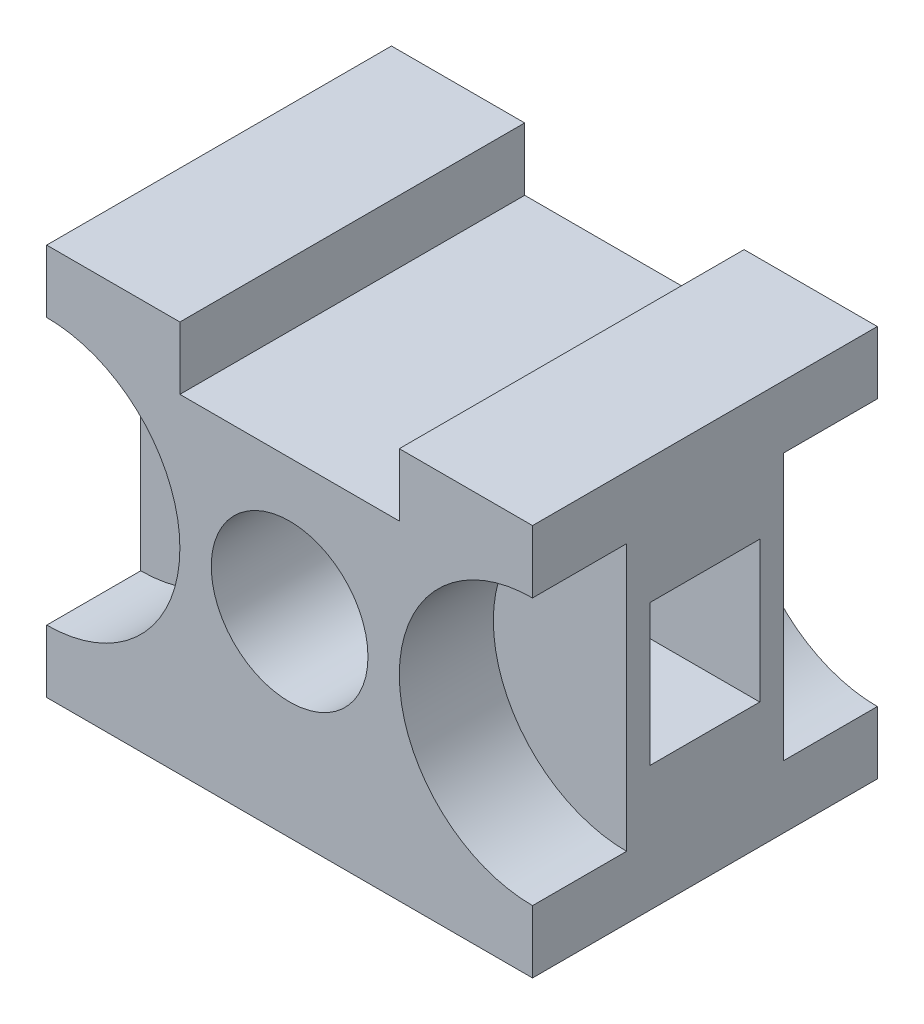
ISO-10303-21;
HEADER;
FILE_DESCRIPTION(('STEP AP214'),'2;1');
FILE_NAME('part.step','',(''),(''),'','','');
FILE_SCHEMA(('AUTOMOTIVE_DESIGN { 1 0 10303 214 1 1 1 1 }'));
ENDSEC;
DATA;
#1=APPLICATION_CONTEXT('core data for automotive mechanical design processes');
#2=APPLICATION_PROTOCOL_DEFINITION('international standard','automotive_design',2000,#1);
#3=PRODUCT_CONTEXT('',#1,'mechanical');
#4=PRODUCT('Part','Part','',(#3));
#5=PRODUCT_RELATED_PRODUCT_CATEGORY('part','',(#4));
#6=PRODUCT_DEFINITION_FORMATION('','',#4);
#7=PRODUCT_DEFINITION_CONTEXT('part definition',#1,'design');
#8=PRODUCT_DEFINITION('design','',#6,#7);
#9=PRODUCT_DEFINITION_SHAPE('','',#8);
#10=(LENGTH_UNIT() NAMED_UNIT(*) SI_UNIT(.MILLI.,.METRE.));
#11=(NAMED_UNIT(*) PLANE_ANGLE_UNIT() SI_UNIT($,.RADIAN.));
#12=(NAMED_UNIT(*) SI_UNIT($,.STERADIAN.) SOLID_ANGLE_UNIT());
#13=UNCERTAINTY_MEASURE_WITH_UNIT(LENGTH_MEASURE(1.E-05),#10,'distance_accuracy_value','');
#14=(GEOMETRIC_REPRESENTATION_CONTEXT(3) GLOBAL_UNCERTAINTY_ASSIGNED_CONTEXT((#13)) GLOBAL_UNIT_ASSIGNED_CONTEXT((#10,
#11,#12)) REPRESENTATION_CONTEXT('',''));
#15=CARTESIAN_POINT('',(0.,0.,0.));
#16=DIRECTION('',(0.,0.,1.));
#17=DIRECTION('',(1.,0.,0.));
#18=AXIS2_PLACEMENT_3D('',#15,#16,#17);
#19=CARTESIAN_POINT('',(-31.,25.,44.));
#20=DIRECTION('',(0.,-1.,0.));
#21=DIRECTION('',(0.,0.,-1.));
#22=AXIS2_PLACEMENT_3D('',#19,#20,#21);
#23=PLANE('',#22);
#24=DIRECTION('',(0.,0.,-1.));
#25=VECTOR('',#24,1.);
#26=CARTESIAN_POINT('',(14.,25.,172.743131660773));
#27=LINE('',#26,#25);
#28=CARTESIAN_POINT('',(14.,25.,44.));
#29=VERTEX_POINT('',#28);
#30=CARTESIAN_POINT('',(14.,25.,0.));
#31=VERTEX_POINT('',#30);
#32=EDGE_CURVE('E272',#29,#31,#27,.T.);
#33=ORIENTED_EDGE('',*,*,#32,.F.);
#34=DIRECTION('',(-1.,0.,0.));
#35=VECTOR('',#34,1.);
#36=CARTESIAN_POINT('',(-31.,25.,44.));
#37=LINE('',#36,#35);
#38=CARTESIAN_POINT('',(31.,25.,44.));
#39=VERTEX_POINT('',#38);
#40=EDGE_CURVE('E323',#39,#29,#37,.T.);
#41=ORIENTED_EDGE('',*,*,#40,.F.);
#42=DIRECTION('',(0.,0.,-1.));
#43=VECTOR('',#42,1.);
#44=CARTESIAN_POINT('',(31.,25.,44.));
#45=LINE('',#44,#43);
#46=CARTESIAN_POINT('',(31.,25.,0.));
#47=VERTEX_POINT('',#46);
#48=EDGE_CURVE('E358',#39,#47,#45,.T.);
#49=ORIENTED_EDGE('',*,*,#48,.T.);
#50=DIRECTION('',(-1.,0.,0.));
#51=VECTOR('',#50,1.);
#52=CARTESIAN_POINT('',(-31.,25.,0.));
#53=LINE('',#52,#51);
#54=EDGE_CURVE('E339',#47,#31,#53,.T.);
#55=ORIENTED_EDGE('',*,*,#54,.T.);
#56=EDGE_LOOP('',(#33,#41,#49,#55));
#57=FACE_BOUND('',#56,.T.);
#58=ADVANCED_FACE('F39',(#57),#23,.F.);
#59=CARTESIAN_POINT('',(0.,0.,44.));
#60=DIRECTION('',(0.,0.,-1.));
#61=DIRECTION('',(-1.,0.,0.));
#62=AXIS2_PLACEMENT_3D('',#59,#60,#61);
#63=PLANE('',#62);
#64=CARTESIAN_POINT('',(0.,0.,44.));
#65=DIRECTION('',(0.,0.,1.));
#66=DIRECTION('',(1.,0.,0.));
#67=AXIS2_PLACEMENT_3D('',#64,#65,#66);
#68=CIRCLE('',#67,10.);
#69=CARTESIAN_POINT('',(10.,0.,44.));
#70=VERTEX_POINT('',#69);
#71=EDGE_CURVE('E311',#70,#70,#68,.T.);
#72=ORIENTED_EDGE('',*,*,#71,.F.);
#73=EDGE_LOOP('',(#72));
#74=FACE_BOUND('',#73,.T.);
#75=DIRECTION('',(0.,-1.,0.));
#76=VECTOR('',#75,1.);
#77=CARTESIAN_POINT('',(-14.,0.,44.));
#78=LINE('',#77,#76);
#79=CARTESIAN_POINT('',(-14.,25.,44.));
#80=VERTEX_POINT('',#79);
#81=CARTESIAN_POINT('',(-14.,17.,44.));
#82=VERTEX_POINT('',#81);
#83=EDGE_CURVE('E281',#80,#82,#78,.T.);
#84=ORIENTED_EDGE('',*,*,#83,.F.);
#85=CARTESIAN_POINT('',(-31.,25.,44.));
#86=VERTEX_POINT('',#85);
#87=EDGE_CURVE('E324',#80,#86,#37,.T.);
#88=ORIENTED_EDGE('',*,*,#87,.T.);
#89=DIRECTION('',(0.,-1.,0.));
#90=VECTOR('',#89,1.);
#91=CARTESIAN_POINT('',(-31.,-25.,44.));
#92=LINE('',#91,#90);
#93=CARTESIAN_POINT('',(-31.,17.,44.));
#94=VERTEX_POINT('',#93);
#95=EDGE_CURVE('E330',#86,#94,#92,.T.);
#96=ORIENTED_EDGE('',*,*,#95,.T.);
#97=CARTESIAN_POINT('',(-31.,0.,44.));
#98=DIRECTION('',(0.,0.,1.));
#99=DIRECTION('',(-1.,0.,0.));
#100=AXIS2_PLACEMENT_3D('',#97,#98,#99);
#101=CIRCLE('',#100,17.);
#102=CARTESIAN_POINT('',(-31.,-17.,44.));
#103=VERTEX_POINT('',#102);
#104=EDGE_CURVE('E286',#103,#94,#101,.T.);
#105=ORIENTED_EDGE('',*,*,#104,.F.);
#106=CARTESIAN_POINT('',(-31.,-25.,44.));
#107=VERTEX_POINT('',#106);
#108=EDGE_CURVE('E327',#103,#107,#92,.T.);
#109=ORIENTED_EDGE('',*,*,#108,.T.);
#110=DIRECTION('',(1.,0.,0.));
#111=VECTOR('',#110,1.);
#112=CARTESIAN_POINT('',(-31.,-25.,44.));
#113=LINE('',#112,#111);
#114=CARTESIAN_POINT('',(31.,-25.,44.));
#115=VERTEX_POINT('',#114);
#116=EDGE_CURVE('E331',#107,#115,#113,.T.);
#117=ORIENTED_EDGE('',*,*,#116,.T.);
#118=DIRECTION('',(0.,1.,0.));
#119=VECTOR('',#118,1.);
#120=CARTESIAN_POINT('',(31.,-25.,44.));
#121=LINE('',#120,#119);
#122=CARTESIAN_POINT('',(31.,-17.,44.));
#123=VERTEX_POINT('',#122);
#124=EDGE_CURVE('E318',#115,#123,#121,.T.);
#125=ORIENTED_EDGE('',*,*,#124,.T.);
#126=CARTESIAN_POINT('',(31.,0.,44.));
#127=DIRECTION('',(0.,0.,1.));
#128=DIRECTION('',(1.,0.,0.));
#129=AXIS2_PLACEMENT_3D('',#126,#127,#128);
#130=CIRCLE('',#129,17.);
#131=CARTESIAN_POINT('',(31.,17.,44.));
#132=VERTEX_POINT('',#131);
#133=EDGE_CURVE('E296',#132,#123,#130,.T.);
#134=ORIENTED_EDGE('',*,*,#133,.F.);
#135=EDGE_CURVE('E321',#132,#39,#121,.T.);
#136=ORIENTED_EDGE('',*,*,#135,.T.);
#137=ORIENTED_EDGE('',*,*,#40,.T.);
#138=DIRECTION('',(0.,1.,0.));
#139=VECTOR('',#138,1.);
#140=CARTESIAN_POINT('',(14.,0.,44.));
#141=LINE('',#140,#139);
#142=CARTESIAN_POINT('',(14.,17.,44.));
#143=VERTEX_POINT('',#142);
#144=EDGE_CURVE('E283',#143,#29,#141,.T.);
#145=ORIENTED_EDGE('',*,*,#144,.F.);
#146=DIRECTION('',(1.,0.,0.));
#147=VECTOR('',#146,1.);
#148=CARTESIAN_POINT('',(0.,17.,44.));
#149=LINE('',#148,#147);
#150=EDGE_CURVE('E282',#82,#143,#149,.T.);
#151=ORIENTED_EDGE('',*,*,#150,.F.);
#152=EDGE_LOOP('',(#84,#88,#96,#105,#109,#117,#125,#134,#136,#137,#145,#151));
#153=FACE_BOUND('',#152,.T.);
#154=ADVANCED_FACE('F408',(#74,#153),#63,.F.);
#155=CARTESIAN_POINT('',(0.,0.,0.));
#156=DIRECTION('',(0.,0.,-1.));
#157=DIRECTION('',(-1.,0.,0.));
#158=AXIS2_PLACEMENT_3D('',#155,#156,#157);
#159=PLANE('',#158);
#160=CARTESIAN_POINT('',(31.,0.,0.));
#161=DIRECTION('',(0.,0.,-1.));
#162=DIRECTION('',(-1.,0.,0.));
#163=AXIS2_PLACEMENT_3D('',#160,#161,#162);
#164=CIRCLE('',#163,17.);
#165=CARTESIAN_POINT('',(31.,-17.,0.));
#166=VERTEX_POINT('',#165);
#167=CARTESIAN_POINT('',(31.,17.,0.));
#168=VERTEX_POINT('',#167);
#169=EDGE_CURVE('E245',#166,#168,#164,.T.);
#170=ORIENTED_EDGE('',*,*,#169,.F.);
#171=DIRECTION('',(0.,1.,0.));
#172=VECTOR('',#171,1.);
#173=CARTESIAN_POINT('',(31.,-25.,0.));
#174=LINE('',#173,#172);
#175=CARTESIAN_POINT('',(31.,-25.,0.));
#176=VERTEX_POINT('',#175);
#177=EDGE_CURVE('E332',#176,#166,#174,.T.);
#178=ORIENTED_EDGE('',*,*,#177,.F.);
#179=DIRECTION('',(1.,0.,0.));
#180=VECTOR('',#179,1.);
#181=CARTESIAN_POINT('',(-31.,-25.,0.));
#182=LINE('',#181,#180);
#183=CARTESIAN_POINT('',(-31.,-25.,0.));
#184=VERTEX_POINT('',#183);
#185=EDGE_CURVE('E348',#184,#176,#182,.T.);
#186=ORIENTED_EDGE('',*,*,#185,.F.);
#187=DIRECTION('',(0.,-1.,0.));
#188=VECTOR('',#187,1.);
#189=CARTESIAN_POINT('',(-31.,-25.,0.));
#190=LINE('',#189,#188);
#191=CARTESIAN_POINT('',(-31.,-17.,0.));
#192=VERTEX_POINT('',#191);
#193=EDGE_CURVE('E345',#192,#184,#190,.T.);
#194=ORIENTED_EDGE('',*,*,#193,.F.);
#195=CARTESIAN_POINT('',(-31.,0.,0.));
#196=DIRECTION('',(0.,0.,-1.));
#197=DIRECTION('',(-1.,0.,0.));
#198=AXIS2_PLACEMENT_3D('',#195,#196,#197);
#199=CIRCLE('',#198,17.);
#200=CARTESIAN_POINT('',(-31.,17.,0.));
#201=VERTEX_POINT('',#200);
#202=EDGE_CURVE('E259',#201,#192,#199,.T.);
#203=ORIENTED_EDGE('',*,*,#202,.F.);
#204=CARTESIAN_POINT('',(-31.,25.,0.));
#205=VERTEX_POINT('',#204);
#206=EDGE_CURVE('E344',#205,#201,#190,.T.);
#207=ORIENTED_EDGE('',*,*,#206,.F.);
#208=CARTESIAN_POINT('',(-14.,25.,0.));
#209=VERTEX_POINT('',#208);
#210=EDGE_CURVE('E336',#209,#205,#53,.T.);
#211=ORIENTED_EDGE('',*,*,#210,.F.);
#212=DIRECTION('',(0.,-1.,0.));
#213=VECTOR('',#212,1.);
#214=CARTESIAN_POINT('',(-14.,0.,0.));
#215=LINE('',#214,#213);
#216=CARTESIAN_POINT('',(-14.,17.,0.));
#217=VERTEX_POINT('',#216);
#218=EDGE_CURVE('E362',#209,#217,#215,.T.);
#219=ORIENTED_EDGE('',*,*,#218,.T.);
#220=DIRECTION('',(1.,0.,0.));
#221=VECTOR('',#220,1.);
#222=CARTESIAN_POINT('',(0.,17.,0.));
#223=LINE('',#222,#221);
#224=CARTESIAN_POINT('',(14.,17.,0.));
#225=VERTEX_POINT('',#224);
#226=EDGE_CURVE('E365',#217,#225,#223,.T.);
#227=ORIENTED_EDGE('',*,*,#226,.T.);
#228=DIRECTION('',(0.,1.,0.));
#229=VECTOR('',#228,1.);
#230=CARTESIAN_POINT('',(14.,0.,0.));
#231=LINE('',#230,#229);
#232=EDGE_CURVE('E360',#225,#31,#231,.T.);
#233=ORIENTED_EDGE('',*,*,#232,.T.);
#234=ORIENTED_EDGE('',*,*,#54,.F.);
#235=EDGE_CURVE('E320',#168,#47,#174,.T.);
#236=ORIENTED_EDGE('',*,*,#235,.F.);
#237=EDGE_LOOP('',(#170,#178,#186,#194,#203,#207,#211,#219,#227,#233,#234,#236));
#238=FACE_BOUND('',#237,.T.);
#239=CARTESIAN_POINT('',(0.,0.,0.));
#240=DIRECTION('',(0.,0.,1.));
#241=DIRECTION('',(1.,0.,0.));
#242=AXIS2_PLACEMENT_3D('',#239,#240,#241);
#243=CIRCLE('',#242,10.);
#244=CARTESIAN_POINT('',(10.,0.,0.));
#245=VERTEX_POINT('',#244);
#246=EDGE_CURVE('E313',#245,#245,#243,.T.);
#247=ORIENTED_EDGE('',*,*,#246,.T.);
#248=EDGE_LOOP('',(#247));
#249=FACE_BOUND('',#248,.T.);
#250=ADVANCED_FACE('F416',(#238,#249),#159,.T.);
#251=CARTESIAN_POINT('',(31.,-25.,44.));
#252=DIRECTION('',(-1.,0.,0.));
#253=DIRECTION('',(0.,0.,1.));
#254=AXIS2_PLACEMENT_3D('',#251,#252,#253);
#255=PLANE('',#254);
#256=DIRECTION('',(0.,0.,1.));
#257=VECTOR('',#256,1.);
#258=CARTESIAN_POINT('',(31.,-9.,15.));
#259=LINE('',#258,#257);
#260=CARTESIAN_POINT('',(31.,-9.,15.));
#261=VERTEX_POINT('',#260);
#262=CARTESIAN_POINT('',(31.,-9.,29.));
#263=VERTEX_POINT('',#262);
#264=EDGE_CURVE('E222',#261,#263,#259,.T.);
#265=ORIENTED_EDGE('',*,*,#264,.T.);
#266=DIRECTION('',(0.,1.,0.));
#267=VECTOR('',#266,1.);
#268=CARTESIAN_POINT('',(31.,9.,29.));
#269=LINE('',#268,#267);
#270=CARTESIAN_POINT('',(31.,9.,29.));
#271=VERTEX_POINT('',#270);
#272=EDGE_CURVE('E209',#263,#271,#269,.T.);
#273=ORIENTED_EDGE('',*,*,#272,.T.);
#274=DIRECTION('',(0.,0.,-1.));
#275=VECTOR('',#274,1.);
#276=CARTESIAN_POINT('',(31.,9.,15.));
#277=LINE('',#276,#275);
#278=CARTESIAN_POINT('',(31.,9.,15.));
#279=VERTEX_POINT('',#278);
#280=EDGE_CURVE('E217',#271,#279,#277,.T.);
#281=ORIENTED_EDGE('',*,*,#280,.T.);
#282=DIRECTION('',(0.,-1.,0.));
#283=VECTOR('',#282,1.);
#284=CARTESIAN_POINT('',(31.,9.,15.));
#285=LINE('',#284,#283);
#286=EDGE_CURVE('E57',#279,#261,#285,.T.);
#287=ORIENTED_EDGE('',*,*,#286,.T.);
#288=EDGE_LOOP('',(#265,#273,#281,#287));
#289=FACE_BOUND('',#288,.T.);
#290=DIRECTION('',(0.,-1.,0.));
#291=VECTOR('',#290,1.);
#292=CARTESIAN_POINT('',(31.,0.,12.));
#293=LINE('',#292,#291);
#294=CARTESIAN_POINT('',(31.,17.,12.));
#295=VERTEX_POINT('',#294);
#296=CARTESIAN_POINT('',(31.,-17.,12.));
#297=VERTEX_POINT('',#296);
#298=EDGE_CURVE('E248',#295,#297,#293,.T.);
#299=ORIENTED_EDGE('',*,*,#298,.F.);
#300=DIRECTION('',(0.,0.,-1.));
#301=VECTOR('',#300,1.);
#302=CARTESIAN_POINT('',(31.,17.,12.));
#303=LINE('',#302,#301);
#304=EDGE_CURVE('E253',#295,#168,#303,.T.);
#305=ORIENTED_EDGE('',*,*,#304,.T.);
#306=ORIENTED_EDGE('',*,*,#235,.T.);
#307=ORIENTED_EDGE('',*,*,#48,.F.);
#308=ORIENTED_EDGE('',*,*,#135,.F.);
#309=DIRECTION('',(0.,0.,1.));
#310=VECTOR('',#309,1.);
#311=CARTESIAN_POINT('',(31.,17.,32.));
#312=LINE('',#311,#310);
#313=CARTESIAN_POINT('',(31.,17.,32.));
#314=VERTEX_POINT('',#313);
#315=EDGE_CURVE('E307',#314,#132,#312,.T.);
#316=ORIENTED_EDGE('',*,*,#315,.F.);
#317=DIRECTION('',(0.,1.,0.));
#318=VECTOR('',#317,1.);
#319=CARTESIAN_POINT('',(31.,17.,32.));
#320=LINE('',#319,#318);
#321=CARTESIAN_POINT('',(31.,-17.,32.));
#322=VERTEX_POINT('',#321);
#323=EDGE_CURVE('E302',#322,#314,#320,.T.);
#324=ORIENTED_EDGE('',*,*,#323,.F.);
#325=DIRECTION('',(0.,0.,1.));
#326=VECTOR('',#325,1.);
#327=CARTESIAN_POINT('',(31.,-17.,32.));
#328=LINE('',#327,#326);
#329=EDGE_CURVE('E310',#322,#123,#328,.T.);
#330=ORIENTED_EDGE('',*,*,#329,.T.);
#331=ORIENTED_EDGE('',*,*,#124,.F.);
#332=DIRECTION('',(0.,0.,-1.));
#333=VECTOR('',#332,1.);
#334=CARTESIAN_POINT('',(31.,-25.,44.));
#335=LINE('',#334,#333);
#336=EDGE_CURVE('E333',#115,#176,#335,.T.);
#337=ORIENTED_EDGE('',*,*,#336,.T.);
#338=ORIENTED_EDGE('',*,*,#177,.T.);
#339=DIRECTION('',(0.,0.,-1.));
#340=VECTOR('',#339,1.);
#341=CARTESIAN_POINT('',(31.,-17.,12.));
#342=LINE('',#341,#340);
#343=EDGE_CURVE('E254',#297,#166,#342,.T.);
#344=ORIENTED_EDGE('',*,*,#343,.F.);
#345=EDGE_LOOP('',(#299,#305,#306,#307,#308,#316,#324,#330,#331,#337,#338,#344));
#346=FACE_BOUND('',#345,.T.);
#347=ADVANCED_FACE('F41',(#289,#346),#255,.F.);
#348=ORIENTED_EDGE('',*,*,#87,.F.);
#349=DIRECTION('',(0.,0.,-1.));
#350=VECTOR('',#349,1.);
#351=CARTESIAN_POINT('',(-14.,25.,172.743131660773));
#352=LINE('',#351,#350);
#353=EDGE_CURVE('E279',#80,#209,#352,.T.);
#354=ORIENTED_EDGE('',*,*,#353,.T.);
#355=ORIENTED_EDGE('',*,*,#210,.T.);
#356=DIRECTION('',(0.,0.,-1.));
#357=VECTOR('',#356,1.);
#358=CARTESIAN_POINT('',(-31.,25.,44.));
#359=LINE('',#358,#357);
#360=EDGE_CURVE('E355',#86,#205,#359,.T.);
#361=ORIENTED_EDGE('',*,*,#360,.F.);
#362=EDGE_LOOP('',(#348,#354,#355,#361));
#363=FACE_BOUND('',#362,.T.);
#364=ADVANCED_FACE('F414',(#363),#23,.F.);
#365=CARTESIAN_POINT('',(-31.,-25.,44.));
#366=DIRECTION('',(1.,0.,0.));
#367=DIRECTION('',(0.,0.,-1.));
#368=AXIS2_PLACEMENT_3D('',#365,#366,#367);
#369=PLANE('',#368);
#370=DIRECTION('',(0.,0.,-1.));
#371=VECTOR('',#370,1.);
#372=CARTESIAN_POINT('',(-31.,9.,15.));
#373=LINE('',#372,#371);
#374=CARTESIAN_POINT('',(-31.,9.,29.));
#375=VERTEX_POINT('',#374);
#376=CARTESIAN_POINT('',(-31.,9.,15.));
#377=VERTEX_POINT('',#376);
#378=EDGE_CURVE('E232',#375,#377,#373,.T.);
#379=ORIENTED_EDGE('',*,*,#378,.F.);
#380=DIRECTION('',(0.,1.,0.));
#381=VECTOR('',#380,1.);
#382=CARTESIAN_POINT('',(-31.,9.,29.));
#383=LINE('',#382,#381);
#384=CARTESIAN_POINT('',(-31.,-9.,29.));
#385=VERTEX_POINT('',#384);
#386=EDGE_CURVE('E61',#385,#375,#383,.T.);
#387=ORIENTED_EDGE('',*,*,#386,.F.);
#388=DIRECTION('',(0.,0.,1.));
#389=VECTOR('',#388,1.);
#390=CARTESIAN_POINT('',(-31.,-9.,15.));
#391=LINE('',#390,#389);
#392=CARTESIAN_POINT('',(-31.,-9.,15.));
#393=VERTEX_POINT('',#392);
#394=EDGE_CURVE('E228',#393,#385,#391,.T.);
#395=ORIENTED_EDGE('',*,*,#394,.F.);
#396=DIRECTION('',(0.,-1.,0.));
#397=VECTOR('',#396,1.);
#398=CARTESIAN_POINT('',(-31.,9.,15.));
#399=LINE('',#398,#397);
#400=EDGE_CURVE('E230',#377,#393,#399,.T.);
#401=ORIENTED_EDGE('',*,*,#400,.F.);
#402=EDGE_LOOP('',(#379,#387,#395,#401));
#403=FACE_BOUND('',#402,.T.);
#404=DIRECTION('',(0.,1.,0.));
#405=VECTOR('',#404,1.);
#406=CARTESIAN_POINT('',(-31.,0.,12.));
#407=LINE('',#406,#405);
#408=CARTESIAN_POINT('',(-31.,-17.,12.));
#409=VERTEX_POINT('',#408);
#410=CARTESIAN_POINT('',(-31.,17.,12.));
#411=VERTEX_POINT('',#410);
#412=EDGE_CURVE('E258',#409,#411,#407,.T.);
#413=ORIENTED_EDGE('',*,*,#412,.F.);
#414=DIRECTION('',(0.,0.,-1.));
#415=VECTOR('',#414,1.);
#416=CARTESIAN_POINT('',(-31.,-17.,12.));
#417=LINE('',#416,#415);
#418=EDGE_CURVE('E269',#409,#192,#417,.T.);
#419=ORIENTED_EDGE('',*,*,#418,.T.);
#420=ORIENTED_EDGE('',*,*,#193,.T.);
#421=DIRECTION('',(0.,0.,-1.));
#422=VECTOR('',#421,1.);
#423=CARTESIAN_POINT('',(-31.,-25.,44.));
#424=LINE('',#423,#422);
#425=EDGE_CURVE('E346',#107,#184,#424,.T.);
#426=ORIENTED_EDGE('',*,*,#425,.F.);
#427=ORIENTED_EDGE('',*,*,#108,.F.);
#428=DIRECTION('',(0.,0.,1.));
#429=VECTOR('',#428,1.);
#430=CARTESIAN_POINT('',(-31.,-17.,32.));
#431=LINE('',#430,#429);
#432=CARTESIAN_POINT('',(-31.,-17.,32.));
#433=VERTEX_POINT('',#432);
#434=EDGE_CURVE('E298',#433,#103,#431,.T.);
#435=ORIENTED_EDGE('',*,*,#434,.F.);
#436=DIRECTION('',(0.,-1.,0.));
#437=VECTOR('',#436,1.);
#438=CARTESIAN_POINT('',(-31.,-17.,32.));
#439=LINE('',#438,#437);
#440=CARTESIAN_POINT('',(-31.,17.,32.));
#441=VERTEX_POINT('',#440);
#442=EDGE_CURVE('E293',#441,#433,#439,.T.);
#443=ORIENTED_EDGE('',*,*,#442,.F.);
#444=DIRECTION('',(0.,0.,1.));
#445=VECTOR('',#444,1.);
#446=CARTESIAN_POINT('',(-31.,17.,32.));
#447=LINE('',#446,#445);
#448=EDGE_CURVE('E295',#441,#94,#447,.T.);
#449=ORIENTED_EDGE('',*,*,#448,.T.);
#450=ORIENTED_EDGE('',*,*,#95,.F.);
#451=ORIENTED_EDGE('',*,*,#360,.T.);
#452=ORIENTED_EDGE('',*,*,#206,.T.);
#453=DIRECTION('',(0.,0.,-1.));
#454=VECTOR('',#453,1.);
#455=CARTESIAN_POINT('',(-31.,17.,12.));
#456=LINE('',#455,#454);
#457=EDGE_CURVE('E265',#411,#201,#456,.T.);
#458=ORIENTED_EDGE('',*,*,#457,.F.);
#459=EDGE_LOOP('',(#413,#419,#420,#426,#427,#435,#443,#449,#450,#451,#452,#458));
#460=FACE_BOUND('',#459,.T.);
#461=ADVANCED_FACE('F395',(#403,#460),#369,.F.);
#462=CARTESIAN_POINT('',(-31.,-25.,44.));
#463=DIRECTION('',(0.,1.,0.));
#464=DIRECTION('',(0.,0.,1.));
#465=AXIS2_PLACEMENT_3D('',#462,#463,#464);
#466=PLANE('',#465);
#467=ORIENTED_EDGE('',*,*,#185,.T.);
#468=ORIENTED_EDGE('',*,*,#336,.F.);
#469=ORIENTED_EDGE('',*,*,#116,.F.);
#470=ORIENTED_EDGE('',*,*,#425,.T.);
#471=EDGE_LOOP('',(#467,#468,#469,#470));
#472=FACE_BOUND('',#471,.T.);
#473=ADVANCED_FACE('F426',(#472),#466,.F.);
#474=CARTESIAN_POINT('',(0.,0.,0.));
#475=DIRECTION('',(0.,0.,1.));
#476=DIRECTION('',(1.,0.,0.));
#477=AXIS2_PLACEMENT_3D('',#474,#475,#476);
#478=CYLINDRICAL_SURFACE('',#477,10.);
#479=DIRECTION('',(0.,0.,1.));
#480=VECTOR('',#479,1.);
#481=CARTESIAN_POINT('',(-4.35889894354067,-9.,0.));
#482=LINE('',#481,#480);
#483=CARTESIAN_POINT('',(-4.35889894354067,-9.,15.));
#484=VERTEX_POINT('',#483);
#485=CARTESIAN_POINT('',(-4.35889894354067,-9.,29.));
#486=VERTEX_POINT('',#485);
#487=EDGE_CURVE('E43',#484,#486,#482,.T.);
#488=ORIENTED_EDGE('',*,*,#487,.T.);
#489=CARTESIAN_POINT('',(0.,0.,29.));
#490=DIRECTION('',(0.,0.,1.));
#491=DIRECTION('',(0.,-1.,0.));
#492=AXIS2_PLACEMENT_3D('',#489,#490,#491);
#493=CIRCLE('',#492,10.);
#494=CARTESIAN_POINT('',(-4.35889894354068,9.,29.));
#495=VERTEX_POINT('',#494);
#496=EDGE_CURVE('E11',#486,#495,#493,.F.);
#497=ORIENTED_EDGE('',*,*,#496,.T.);
#498=DIRECTION('',(0.,0.,1.));
#499=VECTOR('',#498,1.);
#500=CARTESIAN_POINT('',(-4.35889894354068,9.,0.));
#501=LINE('',#500,#499);
#502=CARTESIAN_POINT('',(-4.35889894354068,9.,15.));
#503=VERTEX_POINT('',#502);
#504=EDGE_CURVE('E376',#495,#503,#501,.F.);
#505=ORIENTED_EDGE('',*,*,#504,.T.);
#506=CARTESIAN_POINT('',(0.,0.,15.));
#507=DIRECTION('',(0.,0.,-1.));
#508=DIRECTION('',(0.,1.,0.));
#509=AXIS2_PLACEMENT_3D('',#506,#507,#508);
#510=CIRCLE('',#509,10.);
#511=EDGE_CURVE('E372',#503,#484,#510,.F.);
#512=ORIENTED_EDGE('',*,*,#511,.T.);
#513=EDGE_LOOP('',(#488,#497,#505,#512));
#514=FACE_BOUND('',#513,.T.);
#515=DIRECTION('',(0.,0.,1.));
#516=VECTOR('',#515,1.);
#517=CARTESIAN_POINT('',(4.35889894354068,9.,0.));
#518=LINE('',#517,#516);
#519=CARTESIAN_POINT('',(4.35889894354068,9.,15.));
#520=VERTEX_POINT('',#519);
#521=CARTESIAN_POINT('',(4.35889894354068,9.,29.));
#522=VERTEX_POINT('',#521);
#523=EDGE_CURVE('E368',#520,#522,#518,.T.);
#524=ORIENTED_EDGE('',*,*,#523,.T.);
#525=CARTESIAN_POINT('',(4.35889894354067,-9.,29.));
#526=VERTEX_POINT('',#525);
#527=EDGE_CURVE('E47',#522,#526,#493,.F.);
#528=ORIENTED_EDGE('',*,*,#527,.T.);
#529=DIRECTION('',(0.,0.,1.));
#530=VECTOR('',#529,1.);
#531=CARTESIAN_POINT('',(4.35889894354067,-9.,0.));
#532=LINE('',#531,#530);
#533=CARTESIAN_POINT('',(4.35889894354067,-9.,15.));
#534=VERTEX_POINT('',#533);
#535=EDGE_CURVE('E373',#526,#534,#532,.F.);
#536=ORIENTED_EDGE('',*,*,#535,.T.);
#537=EDGE_CURVE('E369',#534,#520,#510,.F.);
#538=ORIENTED_EDGE('',*,*,#537,.T.);
#539=EDGE_LOOP('',(#524,#528,#536,#538));
#540=FACE_BOUND('',#539,.T.);
#541=ORIENTED_EDGE('',*,*,#246,.F.);
#542=EDGE_LOOP('',(#541));
#543=FACE_BOUND('',#542,.T.);
#544=ORIENTED_EDGE('',*,*,#71,.T.);
#545=EDGE_LOOP('',(#544));
#546=FACE_BOUND('',#545,.T.);
#547=ADVANCED_FACE('F385',(#514,#540,#543,#546),#478,.F.);
#548=CARTESIAN_POINT('',(31.,0.,32.));
#549=DIRECTION('',(0.,0.,1.));
#550=DIRECTION('',(1.,0.,0.));
#551=AXIS2_PLACEMENT_3D('',#548,#549,#550);
#552=CYLINDRICAL_SURFACE('',#551,17.);
#553=ORIENTED_EDGE('',*,*,#133,.T.);
#554=ORIENTED_EDGE('',*,*,#329,.F.);
#555=CARTESIAN_POINT('',(31.,0.,32.));
#556=DIRECTION('',(0.,0.,1.));
#557=DIRECTION('',(1.,0.,0.));
#558=AXIS2_PLACEMENT_3D('',#555,#556,#557);
#559=CIRCLE('',#558,17.);
#560=EDGE_CURVE('E301',#314,#322,#559,.T.);
#561=ORIENTED_EDGE('',*,*,#560,.F.);
#562=ORIENTED_EDGE('',*,*,#315,.T.);
#563=EDGE_LOOP('',(#553,#554,#561,#562));
#564=FACE_BOUND('',#563,.T.);
#565=ADVANCED_FACE('F497',(#564),#552,.F.);
#566=CARTESIAN_POINT('',(31.,0.,32.));
#567=DIRECTION('',(0.,0.,1.));
#568=DIRECTION('',(1.,0.,0.));
#569=AXIS2_PLACEMENT_3D('',#566,#567,#568);
#570=PLANE('',#569);
#571=ORIENTED_EDGE('',*,*,#560,.T.);
#572=ORIENTED_EDGE('',*,*,#323,.T.);
#573=EDGE_LOOP('',(#571,#572));
#574=FACE_BOUND('',#573,.T.);
#575=ADVANCED_FACE('F496',(#574),#570,.T.);
#576=CARTESIAN_POINT('',(-31.,0.,32.));
#577=DIRECTION('',(0.,0.,1.));
#578=DIRECTION('',(1.,0.,0.));
#579=AXIS2_PLACEMENT_3D('',#576,#577,#578);
#580=CYLINDRICAL_SURFACE('',#579,17.);
#581=ORIENTED_EDGE('',*,*,#104,.T.);
#582=ORIENTED_EDGE('',*,*,#448,.F.);
#583=CARTESIAN_POINT('',(-31.,0.,32.));
#584=DIRECTION('',(0.,0.,1.));
#585=DIRECTION('',(-1.,0.,0.));
#586=AXIS2_PLACEMENT_3D('',#583,#584,#585);
#587=CIRCLE('',#586,17.);
#588=EDGE_CURVE('E290',#433,#441,#587,.T.);
#589=ORIENTED_EDGE('',*,*,#588,.F.);
#590=ORIENTED_EDGE('',*,*,#434,.T.);
#591=EDGE_LOOP('',(#581,#582,#589,#590));
#592=FACE_BOUND('',#591,.T.);
#593=ADVANCED_FACE('F458',(#592),#580,.F.);
#594=CARTESIAN_POINT('',(-31.,0.,32.));
#595=DIRECTION('',(0.,0.,-1.));
#596=DIRECTION('',(-1.,0.,0.));
#597=AXIS2_PLACEMENT_3D('',#594,#595,#596);
#598=PLANE('',#597);
#599=ORIENTED_EDGE('',*,*,#588,.T.);
#600=ORIENTED_EDGE('',*,*,#442,.T.);
#601=EDGE_LOOP('',(#599,#600));
#602=FACE_BOUND('',#601,.T.);
#603=ADVANCED_FACE('F457',(#602),#598,.F.);
#604=CARTESIAN_POINT('',(-14.,25.,172.743131660773));
#605=DIRECTION('',(1.,0.,0.));
#606=DIRECTION('',(0.,0.,-1.));
#607=AXIS2_PLACEMENT_3D('',#604,#605,#606);
#608=PLANE('',#607);
#609=ORIENTED_EDGE('',*,*,#353,.F.);
#610=ORIENTED_EDGE('',*,*,#83,.T.);
#611=DIRECTION('',(0.,0.,-1.));
#612=VECTOR('',#611,1.);
#613=CARTESIAN_POINT('',(-14.,17.,172.743131660773));
#614=LINE('',#613,#612);
#615=EDGE_CURVE('E271',#82,#217,#614,.T.);
#616=ORIENTED_EDGE('',*,*,#615,.T.);
#617=ORIENTED_EDGE('',*,*,#218,.F.);
#618=EDGE_LOOP('',(#609,#610,#616,#617));
#619=FACE_BOUND('',#618,.T.);
#620=ADVANCED_FACE('F441',(#619),#608,.T.);
#621=CARTESIAN_POINT('',(-14.,17.,172.743131660773));
#622=DIRECTION('',(0.,1.,0.));
#623=DIRECTION('',(0.,0.,1.));
#624=AXIS2_PLACEMENT_3D('',#621,#622,#623);
#625=PLANE('',#624);
#626=ORIENTED_EDGE('',*,*,#615,.F.);
#627=ORIENTED_EDGE('',*,*,#150,.T.);
#628=DIRECTION('',(0.,0.,-1.));
#629=VECTOR('',#628,1.);
#630=CARTESIAN_POINT('',(14.,17.,172.743131660773));
#631=LINE('',#630,#629);
#632=EDGE_CURVE('E268',#143,#225,#631,.T.);
#633=ORIENTED_EDGE('',*,*,#632,.T.);
#634=ORIENTED_EDGE('',*,*,#226,.F.);
#635=EDGE_LOOP('',(#626,#627,#633,#634));
#636=FACE_BOUND('',#635,.T.);
#637=ADVANCED_FACE('F442',(#636),#625,.T.);
#638=CARTESIAN_POINT('',(14.,17.,172.743131660773));
#639=DIRECTION('',(-1.,0.,0.));
#640=DIRECTION('',(0.,0.,1.));
#641=AXIS2_PLACEMENT_3D('',#638,#639,#640);
#642=PLANE('',#641);
#643=ORIENTED_EDGE('',*,*,#632,.F.);
#644=ORIENTED_EDGE('',*,*,#144,.T.);
#645=ORIENTED_EDGE('',*,*,#32,.T.);
#646=ORIENTED_EDGE('',*,*,#232,.F.);
#647=EDGE_LOOP('',(#643,#644,#645,#646));
#648=FACE_BOUND('',#647,.T.);
#649=ADVANCED_FACE('F477',(#648),#642,.T.);
#650=CARTESIAN_POINT('',(-31.,0.,12.));
#651=DIRECTION('',(0.,0.,-1.));
#652=DIRECTION('',(-1.,0.,0.));
#653=AXIS2_PLACEMENT_3D('',#650,#651,#652);
#654=CYLINDRICAL_SURFACE('',#653,17.);
#655=ORIENTED_EDGE('',*,*,#202,.T.);
#656=ORIENTED_EDGE('',*,*,#418,.F.);
#657=CARTESIAN_POINT('',(-31.,0.,12.));
#658=DIRECTION('',(0.,0.,-1.));
#659=DIRECTION('',(-1.,0.,0.));
#660=AXIS2_PLACEMENT_3D('',#657,#658,#659);
#661=CIRCLE('',#660,17.);
#662=EDGE_CURVE('E264',#411,#409,#661,.T.);
#663=ORIENTED_EDGE('',*,*,#662,.F.);
#664=ORIENTED_EDGE('',*,*,#457,.T.);
#665=EDGE_LOOP('',(#655,#656,#663,#664));
#666=FACE_BOUND('',#665,.T.);
#667=ADVANCED_FACE('F476',(#666),#654,.F.);
#668=CARTESIAN_POINT('',(0.,0.,12.));
#669=DIRECTION('',(0.,0.,-1.));
#670=DIRECTION('',(-1.,0.,0.));
#671=AXIS2_PLACEMENT_3D('',#668,#669,#670);
#672=PLANE('',#671);
#673=ORIENTED_EDGE('',*,*,#412,.T.);
#674=ORIENTED_EDGE('',*,*,#662,.T.);
#675=EDGE_LOOP('',(#673,#674));
#676=FACE_BOUND('',#675,.T.);
#677=ADVANCED_FACE('F488',(#676),#672,.T.);
#678=CARTESIAN_POINT('',(31.,0.,12.));
#679=DIRECTION('',(0.,0.,-1.));
#680=DIRECTION('',(-1.,0.,0.));
#681=AXIS2_PLACEMENT_3D('',#678,#679,#680);
#682=CYLINDRICAL_SURFACE('',#681,17.);
#683=ORIENTED_EDGE('',*,*,#169,.T.);
#684=ORIENTED_EDGE('',*,*,#304,.F.);
#685=CARTESIAN_POINT('',(31.,0.,12.));
#686=DIRECTION('',(0.,0.,-1.));
#687=DIRECTION('',(-1.,0.,0.));
#688=AXIS2_PLACEMENT_3D('',#685,#686,#687);
#689=CIRCLE('',#688,17.);
#690=EDGE_CURVE('E252',#297,#295,#689,.T.);
#691=ORIENTED_EDGE('',*,*,#690,.F.);
#692=ORIENTED_EDGE('',*,*,#343,.T.);
#693=EDGE_LOOP('',(#683,#684,#691,#692));
#694=FACE_BOUND('',#693,.T.);
#695=ADVANCED_FACE('F579',(#694),#682,.F.);
#696=CARTESIAN_POINT('',(0.,0.,12.));
#697=DIRECTION('',(0.,0.,-1.));
#698=DIRECTION('',(-1.,0.,0.));
#699=AXIS2_PLACEMENT_3D('',#696,#697,#698);
#700=PLANE('',#699);
#701=ORIENTED_EDGE('',*,*,#298,.T.);
#702=ORIENTED_EDGE('',*,*,#690,.T.);
#703=EDGE_LOOP('',(#701,#702));
#704=FACE_BOUND('',#703,.T.);
#705=ADVANCED_FACE('F589',(#704),#700,.T.);
#706=CARTESIAN_POINT('',(31.,9.,15.));
#707=DIRECTION('',(0.,1.,0.));
#708=DIRECTION('',(0.,0.,1.));
#709=AXIS2_PLACEMENT_3D('',#706,#707,#708);
#710=PLANE('',#709);
#711=DIRECTION('',(-1.,0.,0.));
#712=VECTOR('',#711,1.);
#713=CARTESIAN_POINT('',(31.,9.,15.));
#714=LINE('',#713,#712);
#715=EDGE_CURVE('E216',#279,#520,#714,.T.);
#716=ORIENTED_EDGE('',*,*,#715,.F.);
#717=ORIENTED_EDGE('',*,*,#280,.F.);
#718=DIRECTION('',(-1.,0.,0.));
#719=VECTOR('',#718,1.);
#720=CARTESIAN_POINT('',(31.,9.,29.));
#721=LINE('',#720,#719);
#722=EDGE_CURVE('E203',#271,#522,#721,.T.);
#723=ORIENTED_EDGE('',*,*,#722,.T.);
#724=ORIENTED_EDGE('',*,*,#523,.F.);
#725=EDGE_LOOP('',(#716,#717,#723,#724));
#726=FACE_BOUND('',#725,.T.);
#727=ADVANCED_FACE('F220',(#726),#710,.F.);
#728=CARTESIAN_POINT('',(31.,9.,15.));
#729=DIRECTION('',(0.,0.,-1.));
#730=DIRECTION('',(0.,1.,0.));
#731=AXIS2_PLACEMENT_3D('',#728,#729,#730);
#732=PLANE('',#731);
#733=DIRECTION('',(-1.,0.,0.));
#734=VECTOR('',#733,1.);
#735=CARTESIAN_POINT('',(31.,-9.,15.));
#736=LINE('',#735,#734);
#737=EDGE_CURVE('E242',#261,#534,#736,.T.);
#738=ORIENTED_EDGE('',*,*,#737,.F.);
#739=ORIENTED_EDGE('',*,*,#286,.F.);
#740=ORIENTED_EDGE('',*,*,#715,.T.);
#741=ORIENTED_EDGE('',*,*,#537,.F.);
#742=EDGE_LOOP('',(#738,#739,#740,#741));
#743=FACE_BOUND('',#742,.T.);
#744=ADVANCED_FACE('F603',(#743),#732,.F.);
#745=CARTESIAN_POINT('',(31.,-9.,15.));
#746=DIRECTION('',(0.,-1.,0.));
#747=DIRECTION('',(0.,0.,-1.));
#748=AXIS2_PLACEMENT_3D('',#745,#746,#747);
#749=PLANE('',#748);
#750=DIRECTION('',(-1.,0.,0.));
#751=VECTOR('',#750,1.);
#752=CARTESIAN_POINT('',(31.,-9.,29.));
#753=LINE('',#752,#751);
#754=EDGE_CURVE('E239',#263,#526,#753,.T.);
#755=ORIENTED_EDGE('',*,*,#754,.F.);
#756=ORIENTED_EDGE('',*,*,#264,.F.);
#757=ORIENTED_EDGE('',*,*,#737,.T.);
#758=ORIENTED_EDGE('',*,*,#535,.F.);
#759=EDGE_LOOP('',(#755,#756,#757,#758));
#760=FACE_BOUND('',#759,.T.);
#761=ADVANCED_FACE('F407',(#760),#749,.F.);
#762=CARTESIAN_POINT('',(31.,9.,29.));
#763=DIRECTION('',(0.,0.,1.));
#764=DIRECTION('',(0.,-1.,0.));
#765=AXIS2_PLACEMENT_3D('',#762,#763,#764);
#766=PLANE('',#765);
#767=ORIENTED_EDGE('',*,*,#722,.F.);
#768=ORIENTED_EDGE('',*,*,#272,.F.);
#769=ORIENTED_EDGE('',*,*,#754,.T.);
#770=ORIENTED_EDGE('',*,*,#527,.F.);
#771=EDGE_LOOP('',(#767,#768,#769,#770));
#772=FACE_BOUND('',#771,.T.);
#773=ADVANCED_FACE('F207',(#772),#766,.F.);
#774=EDGE_CURVE('E243',#486,#385,#753,.T.);
#775=ORIENTED_EDGE('',*,*,#774,.T.);
#776=ORIENTED_EDGE('',*,*,#386,.T.);
#777=EDGE_CURVE('E213',#495,#375,#721,.T.);
#778=ORIENTED_EDGE('',*,*,#777,.F.);
#779=ORIENTED_EDGE('',*,*,#496,.F.);
#780=EDGE_LOOP('',(#775,#776,#778,#779));
#781=FACE_BOUND('',#780,.T.);
#782=ADVANCED_FACE('F400',(#781),#766,.F.);
#783=EDGE_CURVE('E250',#484,#393,#736,.T.);
#784=ORIENTED_EDGE('',*,*,#783,.T.);
#785=ORIENTED_EDGE('',*,*,#394,.T.);
#786=ORIENTED_EDGE('',*,*,#774,.F.);
#787=ORIENTED_EDGE('',*,*,#487,.F.);
#788=EDGE_LOOP('',(#784,#785,#786,#787));
#789=FACE_BOUND('',#788,.T.);
#790=ADVANCED_FACE('F390',(#789),#749,.F.);
#791=EDGE_CURVE('E211',#503,#377,#714,.T.);
#792=ORIENTED_EDGE('',*,*,#791,.T.);
#793=ORIENTED_EDGE('',*,*,#400,.T.);
#794=ORIENTED_EDGE('',*,*,#783,.F.);
#795=ORIENTED_EDGE('',*,*,#511,.F.);
#796=EDGE_LOOP('',(#792,#793,#794,#795));
#797=FACE_BOUND('',#796,.T.);
#798=ADVANCED_FACE('F386',(#797),#732,.F.);
#799=ORIENTED_EDGE('',*,*,#777,.T.);
#800=ORIENTED_EDGE('',*,*,#378,.T.);
#801=ORIENTED_EDGE('',*,*,#791,.F.);
#802=ORIENTED_EDGE('',*,*,#504,.F.);
#803=EDGE_LOOP('',(#799,#800,#801,#802));
#804=FACE_BOUND('',#803,.T.);
#805=ADVANCED_FACE('F396',(#804),#710,.F.);
#806=CLOSED_SHELL('',(#58,#154,#250,#347,#364,#461,#473,#547,#565,#575,#593,#603,#620,#637,#649,
#667,#677,#695,#705,#727,#744,#761,#773,#782,#790,#798,#805));
#807=MANIFOLD_SOLID_BREP('B2',#806);
#808=ADVANCED_BREP_SHAPE_REPRESENTATION('',(#18,#807),#14);
#809=SHAPE_DEFINITION_REPRESENTATION(#9,#808);
ENDSEC;
END-ISO-10303-21;
